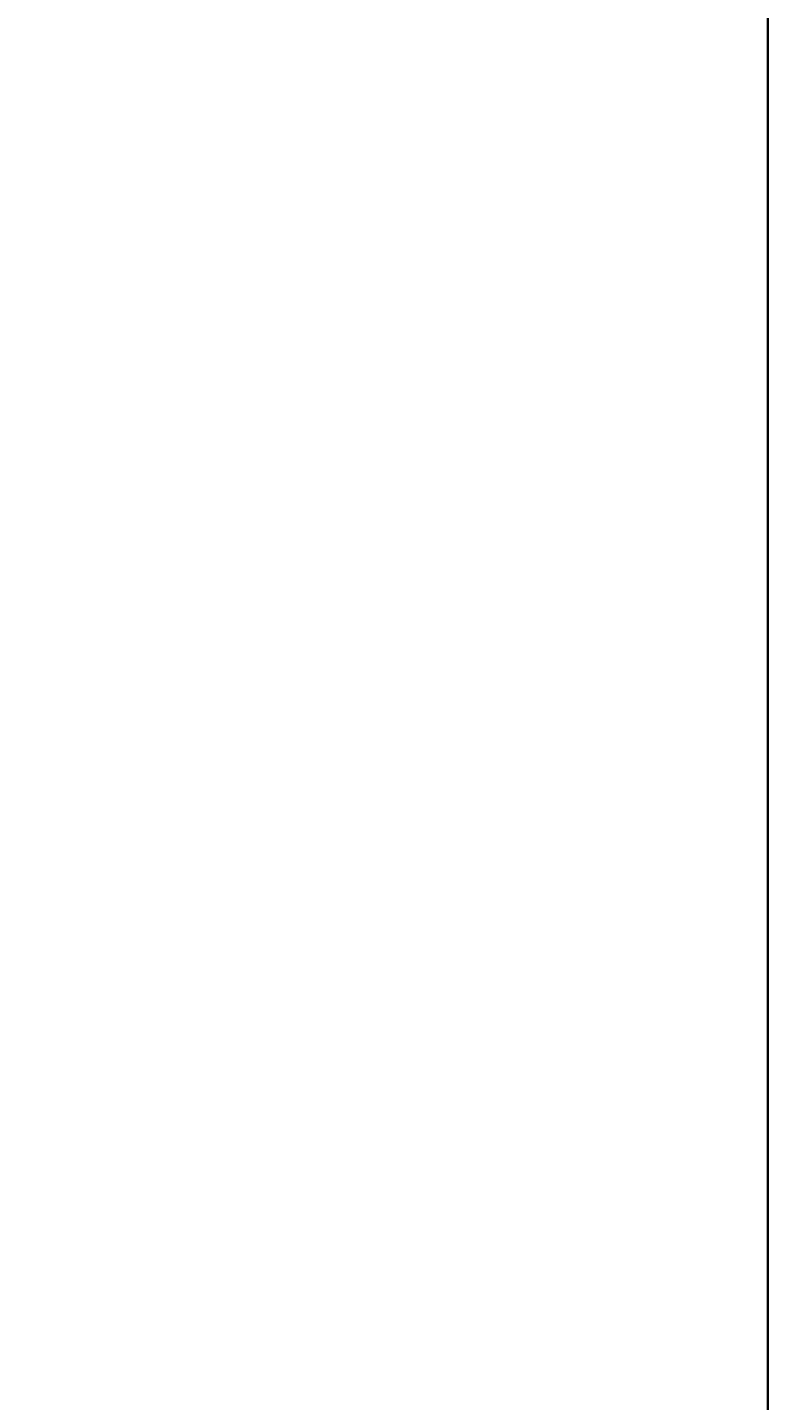
# Model space of a CAD drawing. Units: inches. Extents: x 2163 to 2982, y 1024 to 2288.
# Tile 16 of 22: x 2532 to 2583, y 1885 to 1978. Entities that reach past the tile are written whole.
import ezdxf

# ---------------------------------------------------------------- set-up
doc = ezdxf.new("R2010")
doc.units = ezdxf.units.IN
doc.layers.add('A-ANNO-DIMS', color=2, linetype='Continuous', lineweight=18)
doc.layers.add('A-WALL', color=7, linetype='Continuous', lineweight=35)
doc.styles.get("Standard").update_dxf_attribs({"font": 'arial.ttf'})
doc.dimstyles.get("Standard").update_dxf_attribs({"dimtxt": 0.18, "dimasz": 0.18, "dimexe": 0.18, "dimexo": 0.0625, "dimgap": 0.09, "dimtad": 0, "dimtih": 1, "dimtoh": 1, "dimdec": 4, "dimzin": 0, "dimdsep": 46, "dimtxsty": 'Standard', "dimcen": 0.09, "dimadec": 0, "dimazin": 0, "dimtfac": 1, "dimtdec": 4, "dimtofl": 0, "dimtmove": 0, "dimatfit": 3, "dimfxl": 1, "dimtolj": 1, "dimtzin": 0, "dimarcsym": 0})

# ---------------------------------------------------------------- blocks, each defined once
blk = doc.blocks.new('*D29')
at = {"layer": 'A-ANNO-DIMS', "color": 0, "lineweight": -2, "transparency": 16777216}
for p, q in [((2285.339, 1738.831), (2285.339, 2288.099)), ((2867.339, 2229.331), (2867.339, 2288.099)), ((2285.519, 2287.919), (2576.051, 2287.919)), ((2867.159, 2287.919), (2576.627, 2287.919))]:
    blk.add_line(p, q, dxfattribs=at)
at = {"layer": 'A-ANNO-DIMS', "color": 0, "transparency": 16777216}
for points in [[(2285.519, 2287.949), (2285.519, 2287.889), (2285.339, 2287.919)], [(2867.159, 2287.949), (2867.159, 2287.889), (2867.339, 2287.919)]]:
    blk.add_solid(points, dxfattribs=at)
at = {"layer": 'Defpoints', "color": 0, "transparency": 16777216}
for p in [(2867.339, 2287.919), (2867.339, 2229.269), (2285.339, 1738.769)]:
    blk.add_point(p, dxfattribs=at)
at = {"layer": 'A-ANNO-DIMS', "color": 0, "transparency": 16777216, "insert": (2576.339, 2287.919), "char_height": 0.18, "attachment_point": 5}
blk.add_mtext('\\A1;582', dxfattribs=at)

msp = doc.modelspace()

# ---------------------------------------------------------------- linework, layer by layer
at = {"layer": 'A-WALL'}
msp.add_line((2582.3389, 2011.7688), (2582.3389, 1738.7688), dxfattribs=at)

# ---------------------------------------------------------------- dimensions: what is measured, and where the dimension line sits
at = {"layer": 'A-ANNO-DIMS'}
dim = msp.add_linear_dim(base=(2867.3389, 2287.9188), p1=(2285.3389, 1738.7688), p2=(2867.3389, 2229.2688), dimstyle='Standard', override={"dimdec": 0, "dimlfac": 1, "dimrnd": 0, "dimzin": 0, "dimdsep": 46, "dimlunit": 2}, dxfattribs=at)
dim.commit()
dim.dimension.update_dxf_attribs({"geometry": '*D29', "text_midpoint": (2576.3389, 2287.9188)})

doc.saveas('drawing.dxf')
